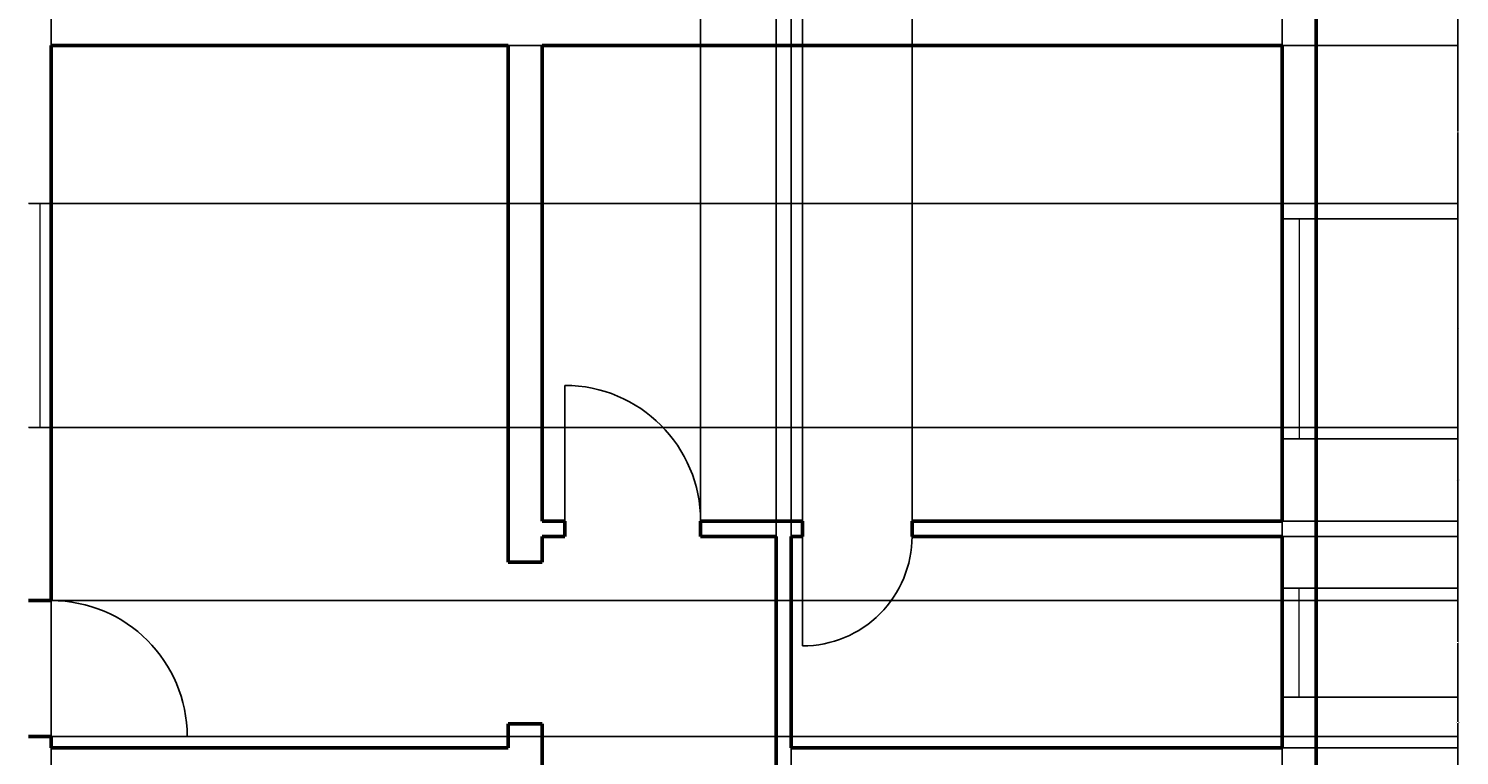
# Model space of a CAD drawing. Units: inches. Extents: x 2479 to 3284, y 2154 to 2936.
# Tile 6 of 8: x 2905 to 3284, y 2346 to 2538. Entities that reach past the tile are written whole.
import ezdxf

# ---------------------------------------------------------------- set-up
doc = ezdxf.new("R2010")
doc.units = ezdxf.units.IN
for name, color, linetype, lineweight in [('A-ANNO-DIMS', 2, 'Continuous', 18), ('A-DOOR', 3, 'Continuous', 25), ('A-GLAZ', 4, 'Continuous', 18), ('A-WALL', 7, 'Continuous', 50)]:
    doc.layers.add(name, color=color, linetype=linetype, lineweight=lineweight)
doc.styles.get("Standard").update_dxf_attribs({"font": 'arial.ttf'})
doc.dimstyles.get("Standard").update_dxf_attribs({"dimtxt": 0.18, "dimasz": 0.18, "dimexe": 0.18, "dimexo": 0.0625, "dimgap": 0.09, "dimtad": 0, "dimtih": 1, "dimtoh": 1, "dimdec": 4, "dimzin": 0, "dimdsep": 46, "dimtxsty": 'Standard', "dimcen": 0.09, "dimadec": 0, "dimazin": 0, "dimtfac": 1, "dimtdec": 4, "dimtofl": 0, "dimtmove": 0, "dimatfit": 3, "dimfxl": 1, "dimtolj": 1, "dimtzin": 0, "dimarcsym": 0})

# ---------------------------------------------------------------- blocks, each defined once
blk = doc.blocks.new('DOOR-SWING-29IN')
blk.add_line((29, 0), (0, 0))
blk.add_arc((29, 0), 29, 90, 180)
blk = doc.blocks.new('DOOR-SWING-36IN')
blk.add_line((36, 0), (0, 0))
blk.add_arc((36, 0), 36, 90, 180)
blk = doc.blocks.new('*D10')
at = {"layer": 'A-ANNO-DIMS', "color": 0, "lineweight": -2, "transparency": 16777216}
for p, q in [((3246.27, 2897.74), (3283.99, 2897.74)), ((3283.81, 2897.56), (3283.81, 2715.92)), ((3283.81, 2533.92), (3283.81, 2715.56)), ((3237.27, 2533.74), (3283.99, 2533.74))]:
    blk.add_line(p, q, dxfattribs=at)
at = {"layer": 'A-ANNO-DIMS', "color": 0, "transparency": 16777216}
for points in [[(3283.78, 2897.56), (3283.84, 2897.56), (3283.81, 2897.74)], [(3283.78, 2533.92), (3283.84, 2533.92), (3283.81, 2533.74)]]:
    blk.add_solid(points, dxfattribs=at)
at = {"layer": 'Defpoints', "color": 0, "transparency": 16777216}
for p in [(3246.21, 2897.74), (3283.81, 2897.74), (3237.21, 2533.74)]:
    blk.add_point(p, dxfattribs=at)
at = {"layer": 'A-ANNO-DIMS', "color": 0, "transparency": 16777216, "insert": (3283.81, 2715.74), "char_height": 0.18, "attachment_point": 5}
blk.add_mtext('\\A1;364', dxfattribs=at)
blk = doc.blocks.new('*D17')
at = {"layer": 'A-ANNO-DIMS', "color": 0, "lineweight": -2, "transparency": 16777216}
for p, q in [((2905.27, 2350.74), (3283.99, 2350.74)), ((3283.81, 2350.56), (3283.81, 2314.42)), ((3283.81, 2277.92), (3283.81, 2314.06)), ((2905.27, 2277.74), (3283.99, 2277.74))]:
    blk.add_line(p, q, dxfattribs=at)
at = {"layer": 'A-ANNO-DIMS', "color": 0, "transparency": 16777216}
for points in [[(3283.78, 2350.56), (3283.84, 2350.56), (3283.81, 2350.74)], [(3283.78, 2277.92), (3283.84, 2277.92), (3283.81, 2277.74)]]:
    blk.add_solid(points, dxfattribs=at)
at = {"layer": 'Defpoints', "color": 0, "transparency": 16777216}
for p in [(2905.21, 2350.74), (3283.81, 2350.74), (2905.21, 2277.74)]:
    blk.add_point(p, dxfattribs=at)
at = {"layer": 'A-ANNO-DIMS', "color": 0, "transparency": 16777216, "insert": (3283.81, 2314.24), "char_height": 0.18, "attachment_point": 5}
blk.add_mtext('\\A1;73', dxfattribs=at)
blk = doc.blocks.new('*D18')
at = {"layer": 'A-ANNO-DIMS', "color": 0, "lineweight": -2, "transparency": 16777216}
for p, q in [((2905.27, 2432.6), (3283.99, 2432.6)), ((3283.81, 2432.42), (3283.81, 2409.85)), ((3283.81, 2386.92), (3283.81, 2409.49)), ((2905.27, 2386.74), (3283.99, 2386.74))]:
    blk.add_line(p, q, dxfattribs=at)
at = {"layer": 'A-ANNO-DIMS', "color": 0, "transparency": 16777216}
for points in [[(3283.78, 2432.42), (3283.84, 2432.42), (3283.81, 2432.6)], [(3283.78, 2386.92), (3283.84, 2386.92), (3283.81, 2386.74)]]:
    blk.add_solid(points, dxfattribs=at)
at = {"layer": 'Defpoints', "color": 0, "transparency": 16777216}
for p in [(2905.21, 2432.6), (3283.81, 2432.6), (2905.21, 2386.74)]:
    blk.add_point(p, dxfattribs=at)
at = {"layer": 'A-ANNO-DIMS', "color": 0, "transparency": 16777216, "insert": (3283.81, 2409.67), "char_height": 0.18, "attachment_point": 5}
blk.add_mtext('\\A1;45.86', dxfattribs=at)
blk = doc.blocks.new('*D19')
at = {"layer": 'A-ANNO-DIMS', "color": 0, "lineweight": -2, "transparency": 16777216}
for p, q in [((2905.27, 2491.94), (3283.99, 2491.94)), ((3283.81, 2491.76), (3283.81, 2462.45)), ((3283.81, 2432.78), (3283.81, 2462.09)), ((2905.27, 2432.6), (3283.99, 2432.6))]:
    blk.add_line(p, q, dxfattribs=at)
at = {"layer": 'A-ANNO-DIMS', "color": 0, "transparency": 16777216}
for points in [[(3283.78, 2491.76), (3283.84, 2491.76), (3283.81, 2491.94)], [(3283.78, 2432.78), (3283.84, 2432.78), (3283.81, 2432.6)]]:
    blk.add_solid(points, dxfattribs=at)
at = {"layer": 'Defpoints', "color": 0, "transparency": 16777216}
for p in [(2905.21, 2491.94), (3283.81, 2491.94), (2905.21, 2432.6)]:
    blk.add_point(p, dxfattribs=at)
at = {"layer": 'A-ANNO-DIMS', "color": 0, "transparency": 16777216, "insert": (3283.81, 2462.27), "char_height": 0.18, "attachment_point": 5}
blk.add_mtext('\\A1;59.33', dxfattribs=at)
blk = doc.blocks.new('*D20')
at = {"layer": 'A-ANNO-DIMS', "color": 0, "lineweight": -2, "transparency": 16777216}
for p, q in [((2911.27, 2542.74), (3283.99, 2542.74)), ((3283.81, 2542.56), (3283.81, 2538.42)), ((3283.81, 2533.92), (3283.81, 2538.06)), ((2911.27, 2533.74), (3283.99, 2533.74))]:
    blk.add_line(p, q, dxfattribs=at)
at = {"layer": 'A-ANNO-DIMS', "color": 0, "transparency": 16777216}
for points in [[(3283.78, 2542.56), (3283.84, 2542.56), (3283.81, 2542.74)], [(3283.78, 2533.92), (3283.84, 2533.92), (3283.81, 2533.74)]]:
    blk.add_solid(points, dxfattribs=at)
at = {"layer": 'Defpoints', "color": 0, "transparency": 16777216}
for p in [(2911.21, 2542.74), (3283.81, 2542.74), (2911.21, 2533.74)]:
    blk.add_point(p, dxfattribs=at)
at = {"layer": 'A-ANNO-DIMS', "color": 0, "transparency": 16777216, "insert": (3283.81, 2538.24), "char_height": 0.18, "attachment_point": 5}
blk.add_mtext('\\A1;9', dxfattribs=at)
blk = doc.blocks.new('*D87')
at = {"layer": 'A-ANNO-DIMS', "color": 0, "lineweight": -2, "transparency": 16777216}
for p, q in [((2911.21, 2542.68), (2911.21, 2153.96)), ((3103.21, 2542.68), (3103.21, 2153.96)), ((2911.39, 2154.14), (3006.93, 2154.14)), ((3103.03, 2154.14), (3007.49, 2154.14))]:
    blk.add_line(p, q, dxfattribs=at)
at = {"layer": 'A-ANNO-DIMS', "color": 0, "transparency": 16777216}
for points in [[(2911.39, 2154.17), (2911.39, 2154.11), (2911.21, 2154.14)], [(3103.03, 2154.17), (3103.03, 2154.11), (3103.21, 2154.14)]]:
    blk.add_solid(points, dxfattribs=at)
at = {"layer": 'Defpoints', "color": 0, "transparency": 16777216}
for p in [(2911.21, 2542.74), (3103.21, 2542.74), (3103.21, 2154.14)]:
    blk.add_point(p, dxfattribs=at)
at = {"layer": 'A-ANNO-DIMS', "color": 0, "transparency": 16777216, "insert": (3007.21, 2154.14), "char_height": 0.18, "attachment_point": 5}
blk.add_mtext('\\A1;192', dxfattribs=at)
blk = doc.blocks.new('*D88')
at = {"layer": 'A-ANNO-DIMS', "color": 0, "lineweight": -2, "transparency": 16777216}
for p, q in [((3107.21, 2542.68), (3107.21, 2153.96)), ((3237.21, 2542.68), (3237.21, 2153.96)), ((3107.39, 2154.14), (3171.93, 2154.14)), ((3237.03, 2154.14), (3172.49, 2154.14))]:
    blk.add_line(p, q, dxfattribs=at)
at = {"layer": 'A-ANNO-DIMS', "color": 0, "transparency": 16777216}
for points in [[(3107.39, 2154.17), (3107.39, 2154.11), (3107.21, 2154.14)], [(3237.03, 2154.17), (3237.03, 2154.11), (3237.21, 2154.14)]]:
    blk.add_solid(points, dxfattribs=at)
at = {"layer": 'Defpoints', "color": 0, "transparency": 16777216}
for p in [(3107.21, 2542.74), (3237.21, 2542.74), (3237.21, 2154.14)]:
    blk.add_point(p, dxfattribs=at)
at = {"layer": 'A-ANNO-DIMS', "color": 0, "transparency": 16777216, "insert": (3172.21, 2154.14), "char_height": 0.18, "attachment_point": 5}
blk.add_mtext('\\A1;130', dxfattribs=at)
blk = doc.blocks.new('*D122')
at = {"layer": 'A-ANNO-DIMS', "color": 0, "lineweight": -2, "transparency": 16777216}
for p, q in [((3237.27, 2361.16), (3283.99, 2361.16)), ((3283.81, 2360.98), (3283.81, 2354.63)), ((3283.81, 2347.92), (3283.81, 2354.27)), ((3237.27, 2347.74), (3283.99, 2347.74))]:
    blk.add_line(p, q, dxfattribs=at)
at = {"layer": 'A-ANNO-DIMS', "color": 0, "transparency": 16777216}
for points in [[(3283.78, 2360.98), (3283.84, 2360.98), (3283.81, 2361.16)], [(3283.78, 2347.92), (3283.84, 2347.92), (3283.81, 2347.74)]]:
    blk.add_solid(points, dxfattribs=at)
at = {"layer": 'Defpoints', "color": 0, "transparency": 16777216}
for p in [(3237.21, 2361.16), (3283.81, 2361.16), (3237.21, 2347.74)]:
    blk.add_point(p, dxfattribs=at)
at = {"layer": 'A-ANNO-DIMS', "color": 0, "transparency": 16777216, "insert": (3283.81, 2354.45), "char_height": 0.18, "attachment_point": 5}
blk.add_mtext('\\A1;13.418', dxfattribs=at)
blk = doc.blocks.new('*D123')
at = {"layer": 'A-ANNO-DIMS', "color": 0, "lineweight": -2, "transparency": 16777216}
for p, q in [((3237.27, 2390.04), (3283.99, 2390.04)), ((3283.81, 2389.86), (3283.81, 2375.78)), ((3283.81, 2361.34), (3283.81, 2375.42)), ((3237.27, 2361.16), (3283.99, 2361.16))]:
    blk.add_line(p, q, dxfattribs=at)
at = {"layer": 'A-ANNO-DIMS', "color": 0, "transparency": 16777216}
for points in [[(3283.78, 2389.86), (3283.84, 2389.86), (3283.81, 2390.04)], [(3283.78, 2361.34), (3283.84, 2361.34), (3283.81, 2361.16)]]:
    blk.add_solid(points, dxfattribs=at)
at = {"layer": 'Defpoints', "color": 0, "transparency": 16777216}
for p in [(3237.21, 2390.04), (3283.81, 2390.04), (3237.21, 2361.16)]:
    blk.add_point(p, dxfattribs=at)
at = {"layer": 'A-ANNO-DIMS', "color": 0, "transparency": 16777216, "insert": (3283.81, 2375.6), "char_height": 0.18, "attachment_point": 5}
blk.add_mtext('\\A1;28.88', dxfattribs=at)
blk = doc.blocks.new('*D124')
at = {"layer": 'A-ANNO-DIMS', "color": 0, "lineweight": -2, "transparency": 16777216}
for p, q in [((3237.27, 2403.74), (3283.99, 2403.74)), ((3283.81, 2403.56), (3283.81, 2397.07)), ((3283.81, 2390.22), (3283.81, 2396.71)), ((3237.27, 2390.04), (3283.99, 2390.04))]:
    blk.add_line(p, q, dxfattribs=at)
at = {"layer": 'A-ANNO-DIMS', "color": 0, "transparency": 16777216}
for points in [[(3283.78, 2403.56), (3283.84, 2403.56), (3283.81, 2403.74)], [(3283.78, 2390.22), (3283.84, 2390.22), (3283.81, 2390.04)]]:
    blk.add_solid(points, dxfattribs=at)
at = {"layer": 'Defpoints', "color": 0, "transparency": 16777216}
for p in [(3237.21, 2403.74), (3283.81, 2403.74), (3237.21, 2390.04)]:
    blk.add_point(p, dxfattribs=at)
at = {"layer": 'A-ANNO-DIMS', "color": 0, "transparency": 16777216, "insert": (3283.81, 2396.89), "char_height": 0.18, "attachment_point": 5}
blk.add_mtext('\\A1;13.7', dxfattribs=at)
blk = doc.blocks.new('*D125')
at = {"layer": 'A-ANNO-DIMS', "color": 0, "lineweight": -2, "transparency": 16777216}
for p, q in [((3237.27, 2429.6), (3283.99, 2429.6)), ((3283.81, 2429.42), (3283.81, 2418.85)), ((3283.81, 2407.92), (3283.81, 2418.49)), ((3237.27, 2407.74), (3283.99, 2407.74))]:
    blk.add_line(p, q, dxfattribs=at)
at = {"layer": 'A-ANNO-DIMS', "color": 0, "transparency": 16777216}
for points in [[(3283.78, 2429.42), (3283.84, 2429.42), (3283.81, 2429.6)], [(3283.78, 2407.92), (3283.84, 2407.92), (3283.81, 2407.74)]]:
    blk.add_solid(points, dxfattribs=at)
at = {"layer": 'Defpoints', "color": 0, "transparency": 16777216}
for p in [(3237.21, 2429.6), (3283.81, 2429.6), (3237.21, 2407.74)]:
    blk.add_point(p, dxfattribs=at)
at = {"layer": 'A-ANNO-DIMS', "color": 0, "transparency": 16777216, "insert": (3283.81, 2418.67), "char_height": 0.18, "attachment_point": 5}
blk.add_mtext('\\A1;21.864', dxfattribs=at)
blk = doc.blocks.new('*D126')
at = {"layer": 'A-ANNO-DIMS', "color": 0, "lineweight": -2, "transparency": 16777216}
for p, q in [((3237.27, 2487.86), (3283.99, 2487.86)), ((3283.81, 2487.68), (3283.81, 2458.91)), ((3283.81, 2429.78), (3283.81, 2458.55)), ((3237.27, 2429.6), (3283.99, 2429.6))]:
    blk.add_line(p, q, dxfattribs=at)
at = {"layer": 'A-ANNO-DIMS', "color": 0, "transparency": 16777216}
for points in [[(3283.78, 2487.68), (3283.84, 2487.68), (3283.81, 2487.86)], [(3283.78, 2429.78), (3283.84, 2429.78), (3283.81, 2429.6)]]:
    blk.add_solid(points, dxfattribs=at)
at = {"layer": 'Defpoints', "color": 0, "transparency": 16777216}
for p in [(3237.21, 2487.86), (3283.81, 2487.86), (3237.21, 2429.6)]:
    blk.add_point(p, dxfattribs=at)
at = {"layer": 'A-ANNO-DIMS', "color": 0, "transparency": 16777216, "insert": (3283.81, 2458.73), "char_height": 0.18, "attachment_point": 5}
blk.add_mtext('\\A1;58.26', dxfattribs=at)
blk = doc.blocks.new('*D127')
at = {"layer": 'A-ANNO-DIMS', "color": 0, "lineweight": -2, "transparency": 16777216}
for p, q in [((3237.27, 2533.74), (3283.99, 2533.74)), ((3283.81, 2533.56), (3283.81, 2510.98)), ((3283.81, 2488.04), (3283.81, 2510.62)), ((3237.27, 2487.86), (3283.99, 2487.86))]:
    blk.add_line(p, q, dxfattribs=at)
at = {"layer": 'A-ANNO-DIMS', "color": 0, "transparency": 16777216}
for points in [[(3283.78, 2533.56), (3283.84, 2533.56), (3283.81, 2533.74)], [(3283.78, 2488.04), (3283.84, 2488.04), (3283.81, 2487.86)]]:
    blk.add_solid(points, dxfattribs=at)
at = {"layer": 'Defpoints', "color": 0, "transparency": 16777216}
for p in [(3237.21, 2533.74), (3283.81, 2533.74), (3237.21, 2487.86)]:
    blk.add_point(p, dxfattribs=at)
at = {"layer": 'A-ANNO-DIMS', "color": 0, "transparency": 16777216, "insert": (3283.81, 2510.8), "char_height": 0.18, "attachment_point": 5}
blk.add_mtext('\\A1;45.88', dxfattribs=at)
blk = doc.blocks.new('*D131')
at = {"layer": 'A-ANNO-DIMS', "color": 0, "lineweight": -2, "transparency": 16777216}
for p, q in [((3083.21, 2407.8), (3083.21, 2935.52)), ((3083.39, 2935.34), (3096.49, 2935.34)), ((3110.03, 2935.34), (3096.93, 2935.34)), ((3110.21, 2407.8), (3110.21, 2935.52))]:
    blk.add_line(p, q, dxfattribs=at)
at = {"layer": 'A-ANNO-DIMS', "color": 0, "transparency": 16777216}
for points in [[(3083.39, 2935.37), (3083.39, 2935.31), (3083.21, 2935.34)], [(3110.03, 2935.37), (3110.03, 2935.31), (3110.21, 2935.34)]]:
    blk.add_solid(points, dxfattribs=at)
at = {"layer": 'Defpoints', "color": 0, "transparency": 16777216}
for p in [(3110.21, 2935.34), (3083.21, 2407.74), (3110.21, 2407.74)]:
    blk.add_point(p, dxfattribs=at)
at = {"layer": 'A-ANNO-DIMS', "color": 0, "transparency": 16777216, "insert": (3096.71, 2935.34), "char_height": 0.18, "attachment_point": 5}
blk.add_mtext('\\A1;27', dxfattribs=at)
blk = doc.blocks.new('*D132')
at = {"layer": 'A-ANNO-DIMS', "color": 0, "lineweight": -2, "transparency": 16777216}
for p, q in [((3139.21, 2407.8), (3139.21, 2935.52)), ((3139.39, 2935.34), (3187.99, 2935.34)), ((3237.03, 2935.34), (3188.43, 2935.34)), ((3237.21, 2407.8), (3237.21, 2935.52))]:
    blk.add_line(p, q, dxfattribs=at)
at = {"layer": 'A-ANNO-DIMS', "color": 0, "transparency": 16777216}
for points in [[(3139.39, 2935.37), (3139.39, 2935.31), (3139.21, 2935.34)], [(3237.03, 2935.37), (3237.03, 2935.31), (3237.21, 2935.34)]]:
    blk.add_solid(points, dxfattribs=at)
at = {"layer": 'Defpoints', "color": 0, "transparency": 16777216}
for p in [(3237.21, 2935.34), (3139.21, 2407.74), (3237.21, 2407.74)]:
    blk.add_point(p, dxfattribs=at)
at = {"layer": 'A-ANNO-DIMS', "color": 0, "transparency": 16777216, "insert": (3188.21, 2935.34), "char_height": 0.18, "attachment_point": 5}
blk.add_mtext('\\A1;98', dxfattribs=at)

msp = doc.modelspace()

# ---------------------------------------------------------------- linework, layer by layer
at = {"layer": 'A-GLAZ'}
for p, q in [((2911.2088, 2491.9355), (2905.2088, 2491.9355)), ((2908.2088, 2491.9355), (2908.2088, 2432.6017)), ((3237.2088, 2487.8605), (3246.2088, 2487.8605)), ((3241.7088, 2487.8605), (3241.7088, 2429.6038)), ((2911.2088, 2432.6017), (2905.2088, 2432.6017)), ((3237.2088, 2429.6038), (3246.2088, 2429.6038)), ((3237.2088, 2390.0399), (3246.2088, 2390.0399)), ((3241.7088, 2361.1579), (3241.7088, 2390.0399)), ((3237.2088, 2361.1579), (3246.2088, 2361.1579))]:
    msp.add_line(p, q, dxfattribs=at)
at = {"layer": 'A-WALL'}
for p, q in [((3246.2088, 2191.7397), (3246.2088, 2897.7397)), ((2911.2088, 2533.7397), (2911.2088, 2386.7397)), ((3032.2088, 2533.7397), (2911.2088, 2533.7397)), ((3032.2088, 2533.7397), (3032.2088, 2396.9151)), ((3041.2088, 2533.7397), (3041.2088, 2407.7397)), ((3237.2088, 2533.7397), (3041.2088, 2533.7397)), ((3237.2088, 2407.7397), (3237.2088, 2533.7397)), ((3047.2088, 2407.7397), (3041.2088, 2407.7397)), ((3047.2088, 2407.7397), (3047.2088, 2403.7397)), ((3083.2088, 2407.7397), (3083.2088, 2403.7397)), ((3110.2088, 2407.7397), (3083.2088, 2407.7397)), ((3110.2088, 2403.7397), (3110.2088, 2407.7397)), ((3237.2088, 2407.7397), (3139.2088, 2407.7397)), ((3139.2088, 2403.7397), (3139.2088, 2407.7397)), ((3047.2088, 2403.7397), (3041.2088, 2403.7397)), ((3041.2088, 2403.7397), (3041.2088, 2396.9151)), ((3103.2088, 2403.7397), (3083.2088, 2403.7397)), ((3103.2088, 2403.7397), (3103.2088, 2340.7397)), ((3107.2088, 2403.7397), (3107.2088, 2347.7397)), ((3110.2088, 2403.7397), (3107.2088, 2403.7397)), ((3237.2088, 2403.7397), (3139.2088, 2403.7397)), ((3237.2088, 2347.7397), (3237.2088, 2403.7397)), ((3041.2088, 2396.9151), (3032.2088, 2396.9151)), ((2911.2088, 2386.7397), (2905.2088, 2386.7397)), ((3041.2088, 2354.1045), (3032.2088, 2354.1045)), ((3032.2088, 2354.1045), (3032.2088, 2347.7397)), ((3041.2088, 2354.1045), (3041.2088, 2338.7702)), ((2911.2088, 2350.7397), (2905.2088, 2350.7397)), ((2911.2088, 2350.7397), (2911.2088, 2347.7397)), ((3032.2088, 2347.7397), (2911.2088, 2347.7397)), ((3237.2088, 2347.7397), (3107.2088, 2347.7397))]:
    msp.add_line(p, q, dxfattribs=at)

# ---------------------------------------------------------------- block references
at = {"layer": 'A-DOOR', "rotation": 269.9999999999902}
msp.add_blockref('DOOR-SWING-36IN', (3047.2088, 2443.7397), dxfattribs=at)
at = {"layer": 'A-DOOR', "extrusion": (0, 0, -1), "zscale": -1, "rotation": 90.0000000000009}
msp.add_blockref('DOOR-SWING-29IN', (-3110.2088, 2374.7397), dxfattribs=at)
at = {"layer": 'A-DOOR', "extrusion": (0, 0, -1), "zscale": -1}
msp.add_blockref('DOOR-SWING-36IN', (-2947.2088, 2350.7397), dxfattribs=at)

# ---------------------------------------------------------------- dimensions: what is measured, and where the dimension line sits
at = {"layer": 'A-ANNO-DIMS'}
for base, p1, p2, picture, middle in [((3110.2088, 2935.3397), (3083.2088, 2407.7397), (3110.2088, 2407.7397), '*D131', (3096.7088, 2935.3397)), ((3237.2088, 2935.3397), (3139.2088, 2407.7397), (3237.2088, 2407.7397), '*D132', (3188.2088, 2935.3397)), ((3103.2088, 2154.1397), (2911.2088, 2542.7397), (3103.2088, 2542.7397), '*D87', (3007.2088, 2154.1397)), ((3237.2088, 2154.1397), (3107.2088, 2542.7397), (3237.2088, 2542.7397), '*D88', (3172.2088, 2154.1397))]:
    dim = msp.add_linear_dim(base=base, p1=p1, p2=p2, dimstyle='Standard', override={"dimdec": 0, "dimlfac": 1, "dimrnd": 0, "dimzin": 0, "dimdsep": 46, "dimlunit": 2}, dxfattribs=at)
    dim.commit()
    dim.dimension.update_dxf_attribs({"geometry": picture, "text_midpoint": middle})
for base, p1, p2, override, picture, middle in [((3283.8088, 2897.7397), (3237.2088, 2533.7397), (3246.2088, 2897.7397), {"dimdec": 0, "dimlfac": 1, "dimrnd": 0, "dimzin": 0, "dimdsep": 46, "dimlunit": 2}, '*D10', (3283.8088, 2715.7397)), ((3283.8088, 2542.7397), (2911.2088, 2533.7397), (2911.2088, 2542.7397), {"dimdec": 0, "dimlfac": 1, "dimrnd": 0, "dimzin": 0, "dimdsep": 46, "dimlunit": 2}, '*D20', (3283.8088, 2538.2397)), ((3283.8088, 2533.7397), (3237.2088, 2487.8605), (3237.2088, 2533.7397), {"dimdec": 2, "dimlfac": 1, "dimrnd": 0, "dimzin": 0, "dimdsep": 46, "dimlunit": 2}, '*D127', (3283.8088, 2510.8001)), ((3283.8088, 2491.9355), (2905.2088, 2432.6017), (2905.2088, 2491.9355), {"dimdec": 2, "dimlfac": 1, "dimrnd": 0, "dimzin": 0, "dimdsep": 46, "dimlunit": 2}, '*D19', (3283.8088, 2462.2686)), ((3283.8088, 2487.8605), (3237.2088, 2429.6038), (3237.2088, 2487.8605), {"dimdec": 2, "dimlfac": 1, "dimrnd": 0, "dimzin": 0, "dimdsep": 46, "dimlunit": 2}, '*D126', (3283.8088, 2458.7321)), ((3283.8088, 2432.6017), (2905.2088, 2386.7397), (2905.2088, 2432.6017), {"dimdec": 2, "dimlfac": 1, "dimrnd": 0, "dimzin": 0, "dimdsep": 46, "dimlunit": 2}, '*D18', (3283.8088, 2409.6707)), ((3283.8088, 2429.6038), (3237.2088, 2407.7397), (3237.2088, 2429.6038), {"dimdec": 3, "dimlfac": 1, "dimrnd": 0, "dimzin": 0, "dimdsep": 46, "dimlunit": 2}, '*D125', (3283.8088, 2418.6718)), ((3283.8088, 2403.7397), (3237.2088, 2390.0399), (3237.2088, 2403.7397), {"dimdec": 1, "dimlfac": 1, "dimrnd": 0, "dimzin": 0, "dimdsep": 46, "dimlunit": 2}, '*D124', (3283.8088, 2396.8898)), ((3283.8088, 2390.0399), (3237.2088, 2361.1579), (3237.2088, 2390.0399), {"dimdec": 2, "dimlfac": 1, "dimrnd": 0, "dimzin": 0, "dimdsep": 46, "dimlunit": 2}, '*D123', (3283.8088, 2375.5989)), ((3283.8088, 2361.1579), (3237.2088, 2347.7397), (3237.2088, 2361.1579), {"dimdec": 3, "dimlfac": 1, "dimrnd": 0, "dimzin": 0, "dimdsep": 46, "dimlunit": 2}, '*D122', (3283.8088, 2354.4488)), ((3283.8088, 2350.7397), (2905.2088, 2277.7397), (2905.2088, 2350.7397), {"dimdec": 0, "dimlfac": 1, "dimrnd": 0, "dimzin": 0, "dimdsep": 46, "dimlunit": 2}, '*D17', (3283.8088, 2314.2397))]:
    dim = msp.add_linear_dim(base=base, p1=p1, p2=p2, angle=90, dimstyle='Standard', override=override, dxfattribs=at)
    dim.commit()
    dim.dimension.update_dxf_attribs({"geometry": picture, "text_midpoint": middle})

doc.saveas('drawing.dxf')
